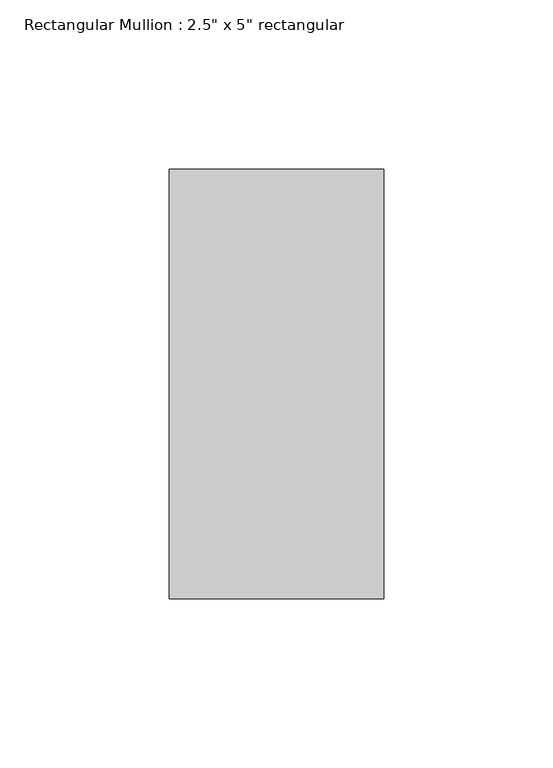
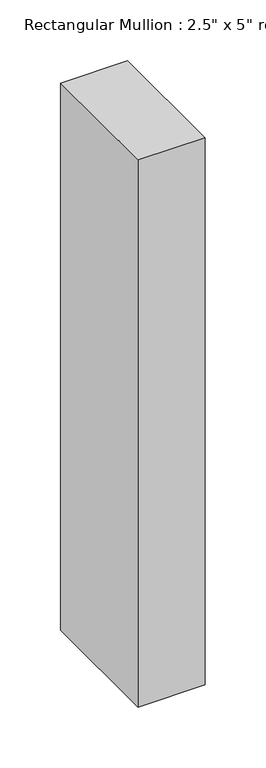
"""IFC4 building model written with IfcOpenShell, lengths in millimetres: member geometry."""

from ifc_helpers import new_model, si_unit, frame, origin, place, context, project, spatial, polyline, outline, extrude, source, transform, mapped, element, save


def member_3683b620(model_context):
    return source(origin(), model_context, "Body", "SweptSolid", [
        extrude(outline(polyline([(31.75, 63.5), (31.75, -63.5), (-31.75, -63.5), (-31.75, 63.5), (31.75, 63.5)])), frame((0.0, 0.0, -548.7736842), z_axis=(0.0, 0.0, 1.0), x_axis=(1.0, 0.0, 0.0)), (0.0, 0.0, 1.0), 548.7736842),
    ])


if __name__ == "__main__":
    model = new_model("IFC4")
    model_context = context("Model", 3, world=origin())
    ifc_project = project(units=[si_unit("LENGTHUNIT", "METRE", prefix="MILLI")], contexts=[model_context])
    site = spatial("IfcSite", under=ifc_project)
    building = spatial("IfcBuilding", under=site)
    placement = place(None, origin())
    member_shape = member_3683b620(model_context)
    element("IfcMember", 1, ObjectType="Rectangular Mullion : 2.5\" x 5\" rectangular", at=placement, inside=building, context=model_context, shape_type="MappedRepresentation", body=[
        mapped(member_shape, transform((0.0, 0.0, 0.0), x_axis=(1.0, 0.0, 0.0), y_axis=(0.0, 1.0, 0.0), z_axis=(0.0, 0.0, 1.0))),
    ])
    save(model, "model.ifc")

# Revit data of these elements
# Type "Rectangular Mullion : 2.5\" x 5\" rectangular"
#   built-in parameter 1007304 = 0.416667 (stored number, unit not read)
#   built-in parameter 1007301 = 0.104167 (stored number, unit not read)
#   built-in parameter 1007300 = 0.104167 (stored number, unit not read)
# Element 1 (IfcMember, "Rectangular Mullion : 2.5\" x 5\" rectangular")
#   Materials on its faces: "Aluminum"
# Materials
#   "Aluminum": class "Metal", colour RGB 247 247 247, transparency 0, Description = "Aluminum 6061", Cost = 0
